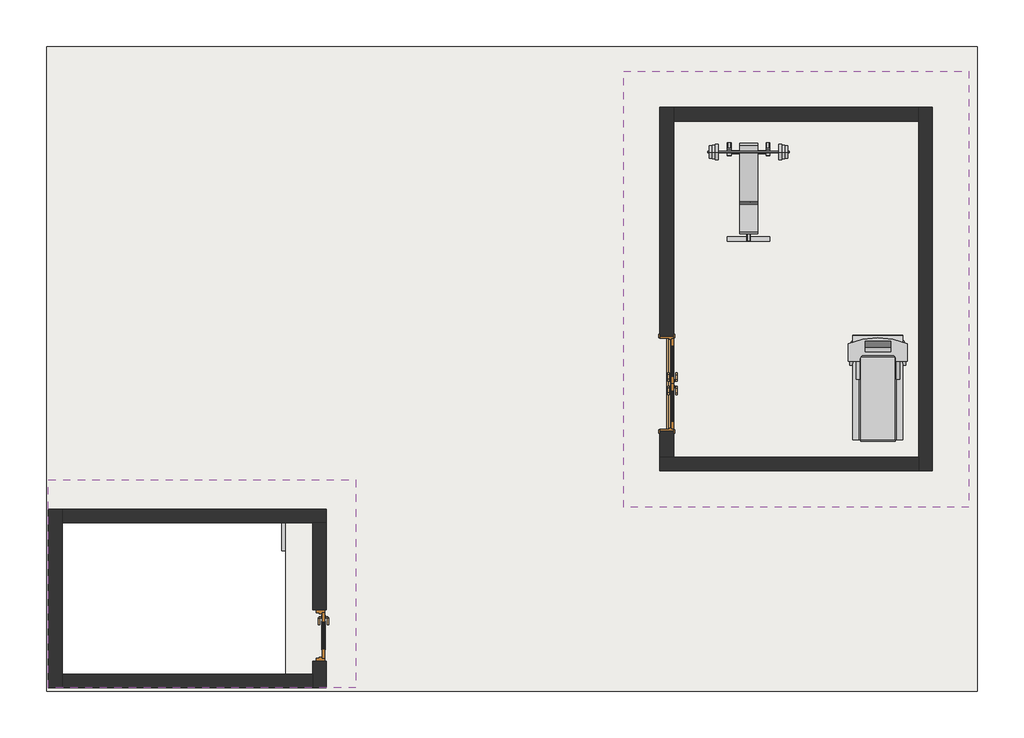
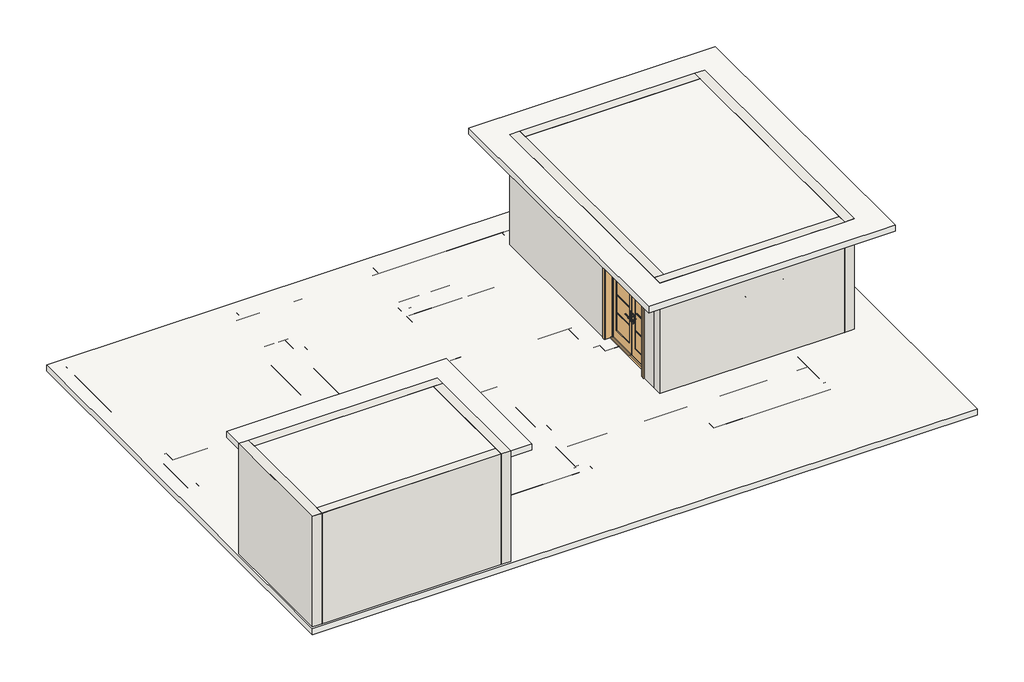
# One storey, incomplete: 18 beams, 8 walls, 3 slabs, 2 doors, 2 proxies.
"""IFC4 building model written with IfcOpenShell, lengths in millimetres."""

from ifc_helpers import new_model, si_unit, frame, origin, place, context, project, spatial, polyline, outline, extrude, faceted_brep, transform, mapped, element, save
from components import lifting_bench_lifting_bench_243d69f3, treadmill_treadmill_b3c1e061, door_7ffae4ec, door_5761e9ac

model = new_model("IFC4")

# Units and contexts
model_context = context("Model", 3, world=origin())
ifc_project = project(units=[si_unit("LENGTHUNIT", "METRE", prefix="MILLI")], contexts=[model_context])

# Site, building, storey
site = spatial("IfcSite", under=ifc_project)
building = spatial("IfcBuilding", under=site)
storey = spatial("IfcBuildingStorey", under=building, Elevation=10210.8)

# Beams
placement = place(None, origin())
element("IfcBeam", 1, ObjectType="Concrete-Rectangular Beam", at=placement, inside=storey, context=model_context, shape_type="Brep", body=[
    faceted_brep([(-8931.9263529, 6644.5661978, 10210.8), (-8931.9263529, 6415.9661978, 10210.8), (-5521.9763529, 6415.9661978, 10210.8), (-5293.3763529, 6415.9661978, 10210.8), (-2264.4263529, 6415.9661978, 10210.8), (-2035.8263529, 6415.9661978, 10210.8), (897.8736471, 6415.9661978, 10210.8), (1126.4736471, 6415.9661978, 10210.8), (3901.4236471, 6415.9661978, 10210.8), (3901.4236471, 6644.5661978, 10210.8), (1164.5736471, 6644.5661978, 10210.8), (1164.5736471, 6454.0661978, 10210.8), (859.7736471, 6454.0661978, 10210.8), (859.7736471, 6644.5661978, 10210.8), (-1997.7263529, 6644.5661978, 10210.8), (-1997.7263529, 6454.0661978, 10210.8), (-2302.5263529, 6454.0661978, 10210.8), (-2302.5263529, 6644.5661978, 10210.8), (-5198.1263529, 6644.5661978, 10210.8), (-5198.1263529, 6454.0661978, 10210.8), (-5502.9263529, 6454.0661978, 10210.8), (-5502.9263529, 6644.5661978, 10210.8), (-8931.9263529, 6415.9661978, 9906.0), (-5521.9763529, 6415.9661978, 9906.0), (-5293.3763529, 6415.9661978, 9906.0), (-2264.4263529, 6415.9661978, 9906.0), (-2035.8263529, 6415.9661978, 9906.0), (897.8736471, 6415.9661978, 9906.0), (1126.4736471, 6415.9661978, 9906.0), (3901.4236471, 6415.9661978, 9906.0), (-8931.9263529, 6644.5661978, 9906.0), (-5502.9263529, 6644.5661978, 9906.0), (-5502.9263529, 6454.0661978, 9906.0), (-5198.1263529, 6454.0661978, 9906.0), (-5198.1263529, 6644.5661978, 9906.0), (-2302.5263529, 6644.5661978, 9906.0), (-2302.5263529, 6454.0661978, 9906.0), (-1997.7263529, 6454.0661978, 9906.0), (-1997.7263529, 6644.5661978, 9906.0), (859.7736471, 6644.5661978, 9906.0), (859.7736471, 6454.0661978, 9906.0), (1164.5736471, 6454.0661978, 9906.0), (1164.5736471, 6644.5661978, 9906.0), (3901.4236471, 6644.5661978, 9906.0)], [[[0, 1, 2, 3, 4, 5, 6, 7, 8, 9, 10, 11, 12, 13, 14, 15, 16, 17, 18, 19, 20, 21]], [[1, 22, 23, 24, 25, 26, 27, 28, 29, 8, 7, 6, 5, 4, 3, 2]], [[22, 30, 31, 32, 33, 34, 35, 36, 37, 38, 39, 40, 41, 42, 43, 29, 28, 27, 26, 25, 24, 23]], [[9, 43, 42, 10]], [[1, 0, 30, 22]], [[9, 8, 29, 43]], [[33, 19, 18, 34]], [[19, 33, 32, 20]], [[20, 32, 31, 21]], [[30, 0, 21, 31]], [[37, 15, 14, 38]], [[15, 37, 36, 16]], [[16, 36, 35, 17]], [[34, 18, 17, 35]], [[41, 11, 10, 42]], [[11, 41, 40, 12]], [[12, 40, 39, 13]], [[38, 14, 13, 39]]]),
])
element("IfcBeam", 2, ObjectType="Concrete-Rectangular Beam", at=placement, inside=storey, context=model_context, shape_type="Brep", body=[
    faceted_brep([(3901.4236471, -1470.7338022, 10210.8), (4130.0236471, -1470.7338022, 10210.8), (4130.0236471, 1748.7161978, 10210.8), (3901.4236471, 1748.7161978, 10210.8), (3901.4236471, 1729.6661978, 10210.8), (3901.4236471, 34.2161978, 10210.8), (3901.4236471, -194.3838022, 10210.8), (3901.4236471, -588.0838022, 10210.8), (3901.4236471, -816.6838022, 10210.8), (3901.4236471, -1470.7338022, 9906.0), (3901.4236471, 1748.7161978, 9906.0), (3901.4236471, 1729.6661978, 9906.0), (3901.4236471, 34.2161978, 9906.0), (3901.4236471, -194.3838022, 9906.0), (3901.4236471, -588.0838022, 9906.0), (3901.4236471, -816.6838022, 9906.0), (4130.0236471, -1470.7338022, 9906.0), (4130.0236471, 1748.7161978, 9906.0)], [[[0, 1, 2, 3, 4, 5, 6, 7, 8]], [[9, 0, 8, 7, 6, 5, 4, 3, 10, 11, 12, 13, 14, 15]], [[16, 9, 15, 14, 13, 12, 11, 10, 17]], [[1, 16, 17, 2]], [[1, 0, 9, 16]], [[3, 2, 17, 10]]]),
    faceted_brep([(3901.4236471, 6377.8661978, 10210.8), (4130.0236471, 6377.8661978, 10210.8), (4130.0236471, 6377.8661978, 9906.0), (3901.4236471, 6377.8661978, 9906.0), (4130.0236471, 2053.5161978, 10210.8), (3901.4236471, 2053.5161978, 10210.8), (3901.4236471, 2053.5161978, 9906.0), (4130.0236471, 2053.5161978, 9906.0), (3901.4236471, 5558.7161978, 10210.8), (3901.4236471, 5330.1161978, 10210.8), (3901.4236471, 5044.3661978, 10210.8), (3901.4236471, 4815.7661978, 10210.8), (3901.4236471, 3012.3661978, 10210.8), (3901.4236471, 2783.7661978, 10210.8), (3901.4236471, 5558.7161978, 9906.0), (3901.4236471, 5330.1161978, 9906.0), (3901.4236471, 5044.3661978, 9906.0), (3901.4236471, 4815.7661978, 9906.0), (3901.4236471, 3012.3661978, 9906.0), (3901.4236471, 2783.7661978, 9906.0)], [[[0, 1, 2, 3]], [[4, 5, 6, 7]], [[1, 0, 8, 9, 10, 11, 12, 13, 5, 4]], [[0, 3, 14, 15, 16, 17, 18, 19, 6, 5, 13, 12, 11, 10, 9, 8]], [[3, 2, 7, 6, 19, 18, 17, 16, 15, 14]], [[2, 1, 4, 7]]]),
])
element("IfcBeam", 3, ObjectType="Concrete-Rectangular Beam", at=placement, inside=storey, context=model_context, shape_type="Brep", body=[
    faceted_brep([(3901.4236471, -1737.4338022, 10210.8), (3901.4236471, -1508.8338022, 10210.8), (-1731.0263529, -1508.8338022, 10210.8), (-1959.6263529, -1508.8338022, 10210.8), (-5293.3763529, -1508.8338022, 10210.8), (-5293.3763529, -1737.4338022, 10210.8), (-1997.7263529, -1737.4338022, 10210.8), (-1997.7263529, -1546.9338022, 10210.8), (-1692.9263529, -1546.9338022, 10210.8), (-1692.9263529, -1737.4338022, 10210.8), (859.7736471, -1737.4338022, 10210.8), (859.7736471, -1546.9338022, 10210.8), (1164.5736471, -1546.9338022, 10210.8), (1164.5736471, -1737.4338022, 10210.8), (3901.4236471, -1508.8338022, 9906.0), (-1731.0263529, -1508.8338022, 9906.0), (-1959.6263529, -1508.8338022, 9906.0), (-5293.3763529, -1508.8338022, 9906.0), (3901.4236471, -1737.4338022, 9906.0), (1164.5736471, -1737.4338022, 9906.0), (1164.5736471, -1546.9338022, 9906.0), (859.7736471, -1546.9338022, 9906.0), (859.7736471, -1737.4338022, 9906.0), (-1692.9263529, -1737.4338022, 9906.0), (-1692.9263529, -1546.9338022, 9906.0), (-1997.7263529, -1546.9338022, 9906.0), (-1997.7263529, -1737.4338022, 9906.0), (-5293.3763529, -1737.4338022, 9906.0)], [[[0, 1, 2, 3, 4, 5, 6, 7, 8, 9, 10, 11, 12, 13]], [[1, 14, 15, 16, 17, 4, 3, 2]], [[14, 18, 19, 20, 21, 22, 23, 24, 25, 26, 27, 17, 16, 15]], [[5, 27, 26, 6]], [[1, 0, 18, 14]], [[5, 4, 17, 27]], [[21, 11, 10, 22]], [[11, 21, 20, 12]], [[12, 20, 19, 13]], [[18, 0, 13, 19]], [[25, 7, 6, 26]], [[7, 25, 24, 8]], [[8, 24, 23, 9]], [[22, 10, 9, 23]]]),
])
element("IfcBeam", 4, ObjectType="Concrete-Rectangular Beam", at=placement, inside=storey, context=model_context, shape_type="Brep", body=[
    faceted_brep([(-5293.3763529, 6415.9661978, 10210.8), (-5521.9763529, 6415.9661978, 10210.8), (-5521.9763529, 3012.3661978, 10210.8), (-5521.9763529, 2783.7661978, 10210.8), (-5521.9763529, 1958.2661978, 10210.8), (-5521.9763529, 1729.6661978, 10210.8), (-5521.9763529, -327.7338022, 10210.8), (-5521.9763529, -556.3338022, 10210.8), (-5521.9763529, -1470.7338022, 10210.8), (-5293.3763529, -1470.7338022, 10210.8), (-5293.3763529, 1729.6661978, 10210.8), (-5401.3263529, 1729.6661978, 10210.8), (-5401.3263529, 1958.2661978, 10210.8), (-5293.3763529, 1958.2661978, 10210.8), (-5293.3763529, 2783.7661978, 10210.8), (-5293.3763529, 3012.3661978, 10210.8), (-5293.3763529, 5330.1161978, 10210.8), (-5293.3763529, 5558.7161978, 10210.8), (-5293.3763529, 6415.9661978, 9906.0), (-5293.3763529, 1958.2661978, 9906.0), (-5293.3763529, 2783.7661978, 9906.0), (-5293.3763529, 3012.3661978, 9906.0), (-5293.3763529, 5330.1161978, 9906.0), (-5293.3763529, 5558.7161978, 9906.0), (-5521.9763529, 6415.9661978, 9906.0), (-5401.3263529, 1958.2661978, 9906.0), (-5401.3263529, 1729.6661978, 9906.0), (-5293.3763529, 1729.6661978, 9906.0), (-5293.3763529, -1470.7338022, 9906.0), (-5521.9763529, -1470.7338022, 9906.0), (-5521.9763529, -556.3338022, 9906.0), (-5521.9763529, -327.7338022, 9906.0), (-5521.9763529, 1729.6661978, 9906.0), (-5521.9763529, 1958.2661978, 9906.0), (-5521.9763529, 2783.7661978, 9906.0), (-5521.9763529, 3012.3661978, 9906.0)], [[[0, 1, 2, 3, 4, 5, 6, 7, 8, 9, 10, 11, 12, 13, 14, 15, 16, 17]], [[18, 0, 17, 16, 15, 14, 13, 19, 20, 21, 22, 23]], [[24, 18, 23, 22, 21, 20, 19, 25, 26, 27, 28, 29, 30, 31, 32, 33, 34, 35]], [[1, 24, 35, 34, 33, 32, 31, 30, 29, 8, 7, 6, 5, 4, 3, 2]], [[1, 0, 18, 24]], [[9, 8, 29, 28]], [[12, 25, 19, 13]], [[26, 11, 10, 27]], [[11, 26, 25, 12]], [[9, 28, 27, 10]]]),
])
element("IfcBeam", 5, ObjectType="Concrete-Rectangular Beam", at=placement, inside=storey, context=model_context, shape_type="SweptSolid", body=[
    extrude(outline(polyline([(-5521.9763529, -327.7338022), (-5521.9763529, -556.3338022), (-8931.9263529, -556.3338022), (-8931.9263529, -327.7338022), (-5521.9763529, -327.7338022)])), frame((0.0, 0.0, 9906.0), z_axis=(0.0, 0.0, 1.0), x_axis=(1.0, 0.0, 0.0)), (0.0, 0.0, 1.0), 304.8),
])
element("IfcBeam", 6, ObjectType="Concrete-Rectangular Beam", at=placement, inside=storey, context=model_context, shape_type="Brep", body=[
    faceted_brep([(-9160.5263529, 6720.7661978, 10210.8), (-8931.9263529, 6720.7661978, 10210.8), (-8931.9263529, 6720.7661978, 9906.0), (-9160.5263529, 6720.7661978, 9906.0), (-9160.5263529, 6682.6661978, 10210.8), (-8931.9263529, 6682.6661978, 10210.8), (-8931.9263529, 6682.6661978, 9906.0), (-9160.5263529, 6682.6661978, 9906.0)], [[[0, 1, 2, 3]], [[1, 0, 4, 5]], [[2, 1, 5, 6]], [[3, 2, 6, 7]], [[0, 3, 7, 4]], [[5, 4, 7, 6]]]),
    faceted_brep([(-8931.9263529, 6377.8661978, 10210.8), (-9160.5263529, 6377.8661978, 10210.8), (-9160.5263529, 3050.4661978, 10210.8), (-8931.9263529, 3050.4661978, 10210.8), (-8931.9263529, 6377.8661978, 9906.0), (-8931.9263529, 3050.4661978, 9906.0), (-9160.5263529, 6377.8661978, 9906.0), (-9160.5263529, 3050.4661978, 9906.0)], [[[0, 1, 2, 3]], [[4, 0, 3, 5]], [[6, 4, 5, 7]], [[1, 6, 7, 2]], [[1, 0, 4, 6]], [[3, 2, 7, 5]]]),
    faceted_brep([(-8931.9263529, -289.6338022, 10210.8), (-9160.5263529, -289.6338022, 10210.8), (-9160.5263529, -289.6338022, 9906.0), (-8931.9263529, -289.6338022, 9906.0), (-9160.5263529, 2745.6661978, 10210.8), (-8931.9263529, 2745.6661978, 10210.8), (-8931.9263529, 2745.6661978, 9906.0), (-9160.5263529, 2745.6661978, 9906.0), (-8931.9263529, 1729.6661978, 10210.8), (-8931.9263529, 1958.2661978, 10210.8), (-8931.9263529, 1729.6661978, 9906.0), (-8931.9263529, 1958.2661978, 9906.0)], [[[0, 1, 2, 3]], [[4, 5, 6, 7]], [[1, 0, 8, 9, 5, 4]], [[0, 3, 10, 11, 6, 5, 9, 8]], [[3, 2, 7, 6, 11, 10]], [[2, 1, 4, 7]]]),
])
element("IfcBeam", 7, ObjectType="Concrete-Rectangular Beam", at=placement, inside=storey, context=model_context, shape_type="Brep", body=[
    faceted_brep([(-8931.9263529, 3012.3661978, 10210.8), (-8931.9263529, 2783.7661978, 10210.8), (-5521.9763529, 2783.7661978, 10210.8), (-5521.9763529, 3012.3661978, 10210.8), (-8931.9263529, 2783.7661978, 9906.0), (-5521.9763529, 2783.7661978, 9906.0), (-8931.9263529, 3012.3661978, 9906.0), (-5521.9763529, 3012.3661978, 9906.0)], [[[0, 1, 2, 3]], [[1, 4, 5, 2]], [[4, 6, 7, 5]], [[6, 0, 3, 7]], [[1, 0, 6, 4]], [[3, 2, 5, 7]]]),
    faceted_brep([(3901.4236471, 3012.3661978, 10210.8), (3901.4236471, 2783.7661978, 10210.8), (3901.4236471, 2783.7661978, 9906.0), (3901.4236471, 3012.3661978, 9906.0), (-5293.3763529, 2783.7661978, 10210.8), (-5293.3763529, 3012.3661978, 10210.8), (-5293.3763529, 3012.3661978, 9906.0), (-5293.3763529, 2783.7661978, 9906.0), (1126.4736471, 3012.3661978, 10210.8), (897.8736471, 3012.3661978, 10210.8), (-2035.8263529, 3012.3661978, 10210.8), (-2264.4263529, 3012.3661978, 10210.8), (-4601.2263529, 3012.3661978, 10210.8), (-4829.8263529, 3012.3661978, 10210.8), (351.7736471, 2783.7661978, 10210.8), (580.3736471, 2783.7661978, 10210.8), (1977.3736471, 2783.7661978, 10210.8), (2205.9736471, 2783.7661978, 10210.8), (351.7736471, 2783.7661978, 9906.0), (580.3736471, 2783.7661978, 9906.0), (1977.3736471, 2783.7661978, 9906.0), (2205.9736471, 2783.7661978, 9906.0), (-4829.8263529, 3012.3661978, 9906.0), (-4601.2263529, 3012.3661978, 9906.0), (-2264.4263529, 3012.3661978, 9906.0), (-2035.8263529, 3012.3661978, 9906.0), (897.8736471, 3012.3661978, 9906.0), (1126.4736471, 3012.3661978, 9906.0)], [[[0, 1, 2, 3]], [[4, 5, 6, 7]], [[1, 0, 8, 9, 10, 11, 12, 13, 5, 4, 14, 15, 16, 17]], [[2, 1, 17, 16, 15, 14, 4, 7, 18, 19, 20, 21]], [[3, 2, 21, 20, 19, 18, 7, 6, 22, 23, 24, 25, 26, 27]], [[0, 3, 27, 26, 25, 24, 23, 22, 6, 5, 13, 12, 11, 10, 9, 8]]]),
])
element("IfcBeam", 8, ObjectType="Concrete-Rectangular Beam", at=placement, inside=storey, context=model_context, shape_type="Brep", body=[
    faceted_brep([(-8931.9263529, 1958.2661978, 10210.8), (-8931.9263529, 1729.6661978, 10210.8), (-5521.9763529, 1729.6661978, 10210.8), (-5521.9763529, 1958.2661978, 10210.8), (-8931.9263529, 1729.6661978, 9906.0), (-5521.9763529, 1729.6661978, 9906.0), (-8931.9263529, 1958.2661978, 9906.0), (-5521.9763529, 1958.2661978, 9906.0)], [[[0, 1, 2, 3]], [[1, 4, 5, 2]], [[4, 6, 7, 5]], [[6, 0, 3, 7]], [[1, 0, 6, 4]], [[3, 2, 5, 7]]]),
    faceted_brep([(3901.4236471, 1958.2661978, 10210.8), (3901.4236471, 1748.7161978, 10210.8), (3901.4236471, 1729.6661978, 10210.8), (3901.4236471, 1729.6661978, 9906.0), (3901.4236471, 1748.7161978, 9906.0), (3901.4236471, 1958.2661978, 9906.0), (618.4736471, 1729.6661978, 10210.8), (618.4736471, 1958.2661978, 10210.8), (618.4736471, 1958.2661978, 9906.0), (618.4736471, 1729.6661978, 9906.0), (2205.9736471, 1958.2661978, 10210.8), (1977.3736471, 1958.2661978, 10210.8), (1977.3736471, 1958.2661978, 9906.0), (2205.9736471, 1958.2661978, 9906.0)], [[[0, 1, 2, 3, 4, 5]], [[6, 7, 8, 9]], [[2, 1, 0, 10, 11, 7, 6]], [[3, 2, 6, 9]], [[5, 4, 3, 9, 8, 12, 13]], [[0, 5, 13, 12, 8, 7, 11, 10]]]),
    faceted_brep([(-5096.5263529, 1958.2661978, 10210.8), (-5096.5263529, 1729.6661978, 10210.8), (-1959.6263529, 1729.6661978, 10210.8), (-1731.0263529, 1729.6661978, 10210.8), (313.6736471, 1729.6661978, 10210.8), (313.6736471, 1958.2661978, 10210.8), (-5096.5263529, 1729.6661978, 9906.0), (-1959.6263529, 1729.6661978, 9906.0), (-1731.0263529, 1729.6661978, 9906.0), (313.6736471, 1729.6661978, 9906.0), (-5096.5263529, 1958.2661978, 9906.0), (313.6736471, 1958.2661978, 9906.0)], [[[0, 1, 2, 3, 4, 5]], [[1, 6, 7, 8, 9, 4, 3, 2]], [[6, 10, 11, 9, 8, 7]], [[10, 0, 5, 11]], [[1, 0, 10, 6]], [[5, 4, 9, 11]]]),
])
element("IfcBeam", 9, ObjectType="Concrete-Rectangular Beam", at=placement, inside=storey, context=model_context, shape_type="Brep", body=[
    faceted_brep([(-1959.6263529, -1508.8338022, 10210.8), (-1731.0263529, -1508.8338022, 10210.8), (-1731.0263529, -816.6838022, 10210.8), (-1731.0263529, -588.0838022, 10210.8), (-1731.0263529, -194.3838022, 10210.8), (-1731.0263529, 34.2161978, 10210.8), (-1731.0263529, 1729.6661978, 10210.8), (-1959.6263529, 1729.6661978, 10210.8), (-1959.6263529, -1508.8338022, 9906.0), (-1959.6263529, 1729.6661978, 9906.0), (-1731.0263529, -1508.8338022, 9906.0), (-1731.0263529, 1729.6661978, 9906.0), (-1731.0263529, 34.2161978, 9906.0), (-1731.0263529, -194.3838022, 9906.0), (-1731.0263529, -588.0838022, 9906.0), (-1731.0263529, -816.6838022, 9906.0)], [[[0, 1, 2, 3, 4, 5, 6, 7]], [[8, 0, 7, 9]], [[10, 8, 9, 11, 12, 13, 14, 15]], [[1, 10, 15, 14, 13, 12, 11, 6, 5, 4, 3, 2]], [[1, 0, 8, 10]], [[7, 6, 11, 9]]]),
])
element("IfcBeam", 10, ObjectType="Concrete-Rectangular Beam", at=placement, inside=storey, context=model_context, shape_type="SweptSolid", body=[
    extrude(outline(polyline([(3901.4236471, -588.0838022), (3901.4236471, -816.6838022), (-1731.0263529, -816.6838022), (-1731.0263529, -588.0838022), (3901.4236471, -588.0838022)])), frame((0.0, 0.0, 9906.0), z_axis=(0.0, 0.0, 1.0), x_axis=(1.0, 0.0, 0.0)), (0.0, 0.0, 1.0), 304.8),
])
element("IfcBeam", 11, ObjectType="Concrete-Rectangular Beam", at=placement, inside=storey, context=model_context, shape_type="SweptSolid", body=[
    extrude(outline(polyline([(3901.4236471, 34.2161978), (3901.4236471, -194.3838022), (-1731.0263529, -194.3838022), (-1731.0263529, 34.2161978), (3901.4236471, 34.2161978)])), frame((0.0, 0.0, 9906.0), z_axis=(0.0, 0.0, 1.0), x_axis=(1.0, 0.0, 0.0)), (0.0, 0.0, 1.0), 304.8),
])
element("IfcBeam", 12, ObjectType="Concrete-Rectangular Beam", at=placement, inside=storey, context=model_context, shape_type="Brep", body=[
    faceted_brep([(3901.4236471, 5330.1161978, 10210.8), (3901.4236471, 5558.7161978, 10210.8), (1126.4736471, 5558.7161978, 10210.8), (897.8736471, 5558.7161978, 10210.8), (-2035.8263529, 5558.7161978, 10210.8), (-2264.4263529, 5558.7161978, 10210.8), (-5293.3763529, 5558.7161978, 10210.8), (-5293.3763529, 5330.1161978, 10210.8), (-4829.8263529, 5330.1161978, 10210.8), (-4601.2263529, 5330.1161978, 10210.8), (-2264.4263529, 5330.1161978, 10210.8), (-2035.8263529, 5330.1161978, 10210.8), (897.8736471, 5330.1161978, 10210.8), (1126.4736471, 5330.1161978, 10210.8), (3901.4236471, 5330.1161978, 9906.0), (-5293.3763529, 5330.1161978, 9906.0), (-4829.8263529, 5330.1161978, 9906.0), (-4601.2263529, 5330.1161978, 9906.0), (-2264.4263529, 5330.1161978, 9906.0), (-2035.8263529, 5330.1161978, 9906.0), (897.8736471, 5330.1161978, 9906.0), (1126.4736471, 5330.1161978, 9906.0), (3901.4236471, 5558.7161978, 9906.0), (-5293.3763529, 5558.7161978, 9906.0), (-2264.4263529, 5558.7161978, 9906.0), (-2035.8263529, 5558.7161978, 9906.0), (897.8736471, 5558.7161978, 9906.0), (1126.4736471, 5558.7161978, 9906.0)], [[[0, 1, 2, 3, 4, 5, 6, 7, 8, 9, 10, 11, 12, 13]], [[14, 0, 13, 12, 11, 10, 9, 8, 7, 15, 16, 17, 18, 19, 20, 21]], [[22, 14, 21, 20, 19, 18, 17, 16, 15, 23, 24, 25, 26, 27]], [[1, 22, 27, 26, 25, 24, 23, 6, 5, 4, 3, 2]], [[1, 0, 14, 22]], [[7, 6, 23, 15]]]),
])
element("IfcBeam", 13, ObjectType="Concrete-Rectangular Beam", at=placement, inside=storey, context=model_context, shape_type="Brep", body=[
    faceted_brep([(3901.4236471, 4815.7661978, 10210.8), (3901.4236471, 5044.3661978, 10210.8), (1126.4736471, 5044.3661978, 10210.8), (897.8736471, 5044.3661978, 10210.8), (-2035.8263529, 5044.3661978, 10210.8), (-2264.4263529, 5044.3661978, 10210.8), (-4601.2263529, 5044.3661978, 10210.8), (-4601.2263529, 4815.7661978, 10210.8), (-2264.4263529, 4815.7661978, 10210.8), (-2035.8263529, 4815.7661978, 10210.8), (897.8736471, 4815.7661978, 10210.8), (1126.4736471, 4815.7661978, 10210.8), (3901.4236471, 4815.7661978, 9906.0), (-4601.2263529, 4815.7661978, 9906.0), (-2264.4263529, 4815.7661978, 9906.0), (-2035.8263529, 4815.7661978, 9906.0), (897.8736471, 4815.7661978, 9906.0), (1126.4736471, 4815.7661978, 9906.0), (3901.4236471, 5044.3661978, 9906.0), (-4601.2263529, 5044.3661978, 9906.0), (-2264.4263529, 5044.3661978, 9906.0), (-2035.8263529, 5044.3661978, 9906.0), (897.8736471, 5044.3661978, 9906.0), (1126.4736471, 5044.3661978, 9906.0)], [[[0, 1, 2, 3, 4, 5, 6, 7, 8, 9, 10, 11]], [[12, 0, 11, 10, 9, 8, 7, 13, 14, 15, 16, 17]], [[18, 12, 17, 16, 15, 14, 13, 19, 20, 21, 22, 23]], [[1, 18, 23, 22, 21, 20, 19, 6, 5, 4, 3, 2]], [[1, 0, 12, 18]], [[7, 6, 19, 13]]]),
])
element("IfcBeam", 14, ObjectType="Concrete-Rectangular Beam", at=placement, inside=storey, context=model_context, shape_type="Brep", body=[
    faceted_brep([(-4829.8263529, 3012.3661978, 10210.8), (-4601.2263529, 3012.3661978, 10210.8), (-4601.2263529, 4815.7661978, 10210.8), (-4601.2263529, 5044.3661978, 10210.8), (-4601.2263529, 5330.1161978, 10210.8), (-4829.8263529, 5330.1161978, 10210.8), (-4829.8263529, 3012.3661978, 9906.0), (-4829.8263529, 5330.1161978, 9906.0), (-4601.2263529, 3012.3661978, 9906.0), (-4601.2263529, 5330.1161978, 9906.0), (-4601.2263529, 5044.3661978, 9906.0), (-4601.2263529, 4815.7661978, 9906.0)], [[[0, 1, 2, 3, 4, 5]], [[6, 0, 5, 7]], [[8, 6, 7, 9, 10, 11]], [[1, 8, 11, 10, 9, 4, 3, 2]], [[1, 0, 6, 8]], [[5, 4, 9, 7]]]),
])
element("IfcBeam", 15, ObjectType="Concrete-Rectangular Beam", at=placement, inside=storey, context=model_context, shape_type="SweptSolid", body=[
    extrude(outline(polyline([(-2035.8263529, 3012.3661978), (-2264.4263529, 3012.3661978), (-2264.4263529, 4815.7661978), (-2035.8263529, 4815.7661978), (-2035.8263529, 3012.3661978)])), frame((0.0, 0.0, 9906.0), z_axis=(0.0, 0.0, 1.0), x_axis=(1.0, 0.0, 0.0)), (0.0, 0.0, 1.0), 304.8),
    extrude(outline(polyline([(-2264.4263529, 6415.9661978), (-2035.8263529, 6415.9661978), (-2035.8263529, 5558.7161978), (-2264.4263529, 5558.7161978), (-2264.4263529, 6415.9661978)])), frame((0.0, 0.0, 9906.0), z_axis=(0.0, 0.0, 1.0), x_axis=(1.0, 0.0, 0.0)), (0.0, 0.0, 1.0), 304.8),
    extrude(outline(polyline([(-2264.4263529, 5330.1161978), (-2035.8263529, 5330.1161978), (-2035.8263529, 5044.3661978), (-2264.4263529, 5044.3661978), (-2264.4263529, 5330.1161978)])), frame((0.0, 0.0, 9906.0), z_axis=(0.0, 0.0, 1.0), x_axis=(1.0, 0.0, 0.0)), (0.0, 0.0, 1.0), 304.8),
])
element("IfcBeam", 16, ObjectType="Concrete-Rectangular Beam", at=placement, inside=storey, context=model_context, shape_type="SweptSolid", body=[
    extrude(outline(polyline([(1126.4736471, 3012.3661978), (897.8736471, 3012.3661978), (897.8736471, 4815.7661978), (1126.4736471, 4815.7661978), (1126.4736471, 3012.3661978)])), frame((0.0, 0.0, 9906.0), z_axis=(0.0, 0.0, 1.0), x_axis=(1.0, 0.0, 0.0)), (0.0, 0.0, 1.0), 304.8),
    extrude(outline(polyline([(897.8736471, 6415.9661978), (1126.4736471, 6415.9661978), (1126.4736471, 5558.7161978), (897.8736471, 5558.7161978), (897.8736471, 6415.9661978)])), frame((0.0, 0.0, 9906.0), z_axis=(0.0, 0.0, 1.0), x_axis=(1.0, 0.0, 0.0)), (0.0, 0.0, 1.0), 304.8),
    extrude(outline(polyline([(897.8736471, 5330.1161978), (1126.4736471, 5330.1161978), (1126.4736471, 5044.3661978), (897.8736471, 5044.3661978), (897.8736471, 5330.1161978)])), frame((0.0, 0.0, 9906.0), z_axis=(0.0, 0.0, 1.0), x_axis=(1.0, 0.0, 0.0)), (0.0, 0.0, 1.0), 304.8),
])
element("IfcBeam", 17, ObjectType="Concrete-Rectangular Beam", at=placement, inside=storey, context=model_context, shape_type="SweptSolid", body=[
    extrude(outline(polyline([(351.7736471, 2783.7661978), (580.3736471, 2783.7661978), (580.3736471, 1958.2661978), (351.7736471, 1958.2661978), (351.7736471, 2783.7661978)])), frame((0.0, 0.0, 9906.0), z_axis=(0.0, 0.0, 1.0), x_axis=(1.0, 0.0, 0.0)), (0.0, 0.0, 1.0), 304.8),
])
element("IfcBeam", 18, ObjectType="Concrete-Rectangular Beam", at=placement, inside=storey, context=model_context, shape_type="SweptSolid", body=[
    extrude(outline(polyline([(1977.3736471, 2783.7661978), (2205.9736471, 2783.7661978), (2205.9736471, 1958.2661978), (1977.3736471, 1958.2661978), (1977.3736471, 2783.7661978)])), frame((0.0, 0.0, 9906.0), z_axis=(0.0, 0.0, 1.0), x_axis=(1.0, 0.0, 0.0)), (0.0, 0.0, 1.0), 304.8),
])

# Proxies
lifting_bench_lifting_bench_shape = lifting_bench_lifting_bench_243d69f3(model_context)
element("IfcBuildingElementProxy", 19, Name="Lifting Bench : Lifting Bench", ObjectType="Lifting Bench : Lifting Bench", at=placement, inside=storey, context=model_context, shape_type="MappedRepresentation", body=[
    mapped(lifting_bench_lifting_bench_shape, transform((1954.8382003, 3718.5744906, 10210.8), x_axis=(1.0, 0.0, 0.0), y_axis=(0.0, 1.0, 0.0), z_axis=(0.0, 0.0, 1.0))),
])
treadmill_treadmill_shape = treadmill_treadmill_b3c1e061(model_context)
element("IfcBuildingElementProxy", 20, Name="Treadmill : Treadmill", ObjectType="Treadmill : Treadmill", at=placement, inside=storey, context=model_context, shape_type="MappedRepresentation", body=[
    mapped(treadmill_treadmill_shape, transform((4035.8856165, 2143.7744906, 10210.8), x_axis=(1.0, 0.0, 0.0), y_axis=(0.0, 1.0, 0.0), z_axis=(0.0, 0.0, 1.0))),
])

# Doors
door_shape = door_7ffae4ec(model_context)
element("IfcDoor", 21, ObjectType="Door-Exterior-Double-Full Glass-Wood_Clad : 60\" x 84\"", at=placement, inside=storey, context=model_context, shape_type="MappedRepresentation", body=[
    mapped(door_shape, transform((940.2606165, 1330.9744906, 10210.8), x_axis=(0.0, -1.0, 0.0), y_axis=(1.0, 0.0, 0.0), z_axis=(0.0, 0.0, 1.0))),
])
door_2_shape = door_5761e9ac(model_context)
element("IfcDoor", 22, ObjectType="Door-Passage-Single-Full_Lite : 30\" x 84\"", at=placement, inside=storey, context=model_context, shape_type="MappedRepresentation", body=[
    mapped(door_2_shape, transform((-4893.3263529, -2893.1338022, 10210.8), x_axis=(0.0, -1.0, 0.0), y_axis=(1.0, 0.0, 0.0), z_axis=(0.0, 0.0, 1.0))),
])

# Slabs
element("IfcSlab", 23, ObjectType="Generic - 6\"", at=placement, inside=storey, context=model_context, shape_type="SweptSolid", body=[
    extrude(outline(polyline([(6149.3236471, 6987.4661978), (6149.3236471, -3826.5838022), (-9465.3263529, -3826.5838022), (-9465.3263529, 6987.4661978), (6149.3236471, 6987.4661978)]), holes=[polyline([(-5458.4763529, -1000.8338022), (-9204.9763529, -1000.8338022), (-9204.9763529, -3540.8338022), (-5458.4763529, -3540.8338022), (-5458.4763529, -1000.8338022)])]), frame((0.0, 0.0, 10058.4), z_axis=(0.0, 0.0, 1.0), x_axis=(1.0, 0.0, 0.0)), (0.0, 0.0, 1.0), 152.4),
])
element("IfcSlab", 24, ObjectType="Generic - 6\"", at=placement, inside=storey, context=model_context, shape_type="SweptSolid", body=[
    extrude(outline(polyline([(-4277.3763529, -3769.4338022), (-9433.5763529, -3769.4338022), (-9433.5763529, -276.9338022), (-4277.3763529, -276.9338022), (-4277.3763529, -3769.4338022)])), frame((0.0, 0.0, 12801.6), z_axis=(0.0, 0.0, 1.0), x_axis=(1.0, 0.0, 0.0)), (0.0, 0.0, 1.0), 152.4),
])
element("IfcSlab", 25, ObjectType="Generic - 6\"", at=placement, inside=storey, context=model_context, shape_type="SweptSolid", body=[
    extrude(outline(polyline([(6004.3856165, 6576.0744906), (6004.3856165, -739.1255094), (213.1856165, -739.1255094), (213.1856165, 6576.0744906), (6004.3856165, 6576.0744906)])), frame((0.0, 0.0, 12801.6), z_axis=(0.0, 0.0, 1.0), x_axis=(1.0, 0.0, 0.0)), (0.0, 0.0, 1.0), 152.4),
])

# Walls
element("IfcWall", 26, ObjectType="Generic - 9\"", at=placement, inside=storey, context=model_context, shape_type="Brep", body=[
    faceted_brep([(-9433.5763529, -772.2338022, 10210.8), (-9433.5763529, -3769.4338022, 10210.8), (-9433.5763529, -3769.4338022, 12954.0), (-9433.5763529, -772.2338022, 12954.0), (-9204.9763529, -772.2338022, 10210.8), (-9204.9763529, -772.2338022, 12954.0), (-9204.9763529, -1000.8338022, 12954.0), (-9204.9763529, -3540.8338022, 12954.0), (-9204.9763529, -3769.4338022, 12954.0), (-9204.9763529, -3769.4338022, 10210.8), (-9204.9763529, -3540.8338022, 10210.8), (-9204.9763529, -1000.8338022, 10210.8)], [[[0, 1, 2, 3]], [[4, 5, 6, 7, 8, 9, 10, 11]], [[1, 0, 4, 11, 10, 9]], [[3, 2, 8, 7, 6, 5]], [[2, 1, 9, 8]], [[0, 3, 5, 4]]]),
])
element("IfcWall", 27, ObjectType="Generic - 9\"", at=placement, inside=storey, context=model_context, shape_type="SweptSolid", body=[
    extrude(outline(polyline([(-5001.2763529, -3769.4338022), (-9204.9763529, -3769.4338022), (-9204.9763529, -3540.8338022), (-5001.2763529, -3540.8338022), (-5001.2763529, -3769.4338022)])), frame((0.0, 0.0, 10210.8), z_axis=(0.0, 0.0, 1.0), x_axis=(1.0, 0.0, 0.0)), (0.0, 0.0, 1.0), 2743.2),
])
element("IfcWall", 28, ObjectType="Generic - 9\"", at=placement, inside=storey, context=model_context, shape_type="Brep", body=[
    faceted_brep([(-9204.9763529, -1000.8338022, 10210.8), (-5001.2763529, -1000.8338022, 10210.8), (-4772.6763529, -1000.8338022, 10210.8), (-4772.6763529, -1000.8338022, 12954.0), (-5001.2763529, -1000.8338022, 12954.0), (-9204.9763529, -1000.8338022, 12954.0), (-9204.9763529, -772.2338022, 10210.8), (-9204.9763529, -772.2338022, 12954.0), (-4772.6763529, -772.2338022, 12954.0), (-4772.6763529, -772.2338022, 10210.8)], [[[0, 1, 2, 3, 4, 5]], [[6, 7, 8, 9]], [[2, 1, 0, 6, 9]], [[5, 4, 3, 8, 7]], [[0, 5, 7, 6]], [[3, 2, 9, 8]]]),
])
element("IfcWall", 29, ObjectType="Generic - 9\"", at=placement, inside=storey, context=model_context, shape_type="Brep", body=[
    faceted_brep([(-5001.2763529, -3769.4338022, 12954.0), (-5001.2763529, -3540.8338022, 12954.0), (-5001.2763529, -1000.8338022, 12954.0), (-5001.2763529, -1000.8338022, 10210.8), (-5001.2763529, -2461.3338022, 10210.8), (-5001.2763529, -2461.3338022, 12446.0), (-5001.2763529, -3324.9338022, 12446.0), (-5001.2763529, -3324.9338022, 10210.8), (-5001.2763529, -3540.8338022, 10210.8), (-5001.2763529, -3769.4338022, 10210.8), (-4772.6763529, -1000.8338022, 12954.0), (-4772.6763529, -3769.4338022, 12954.0), (-4772.6763529, -3769.4338022, 10210.8), (-4772.6763529, -3324.9338022, 10210.8), (-4772.6763529, -3324.9338022, 12446.0), (-4772.6763529, -2461.3338022, 12446.0), (-4772.6763529, -2461.3338022, 10210.8), (-4772.6763529, -1000.8338022, 10210.8)], [[[0, 1, 2, 3, 4, 5, 6, 7, 8, 9]], [[10, 11, 12, 13, 14, 15, 16, 17]], [[3, 17, 16, 4]], [[12, 9, 8, 7, 13]], [[2, 1, 0, 11, 10]], [[3, 2, 10, 17]], [[0, 9, 12, 11]], [[6, 14, 13, 7]], [[14, 6, 5, 15]], [[15, 5, 4, 16]]]),
])
element("IfcWall", 30, ObjectType="Generic - 9\"", at=placement, inside=storey, context=model_context, shape_type="Brep", body=[
    faceted_brep([(5166.1856165, 5966.4744906, 10210.8), (5166.1856165, 5737.8744906, 10210.8), (5166.1856165, 99.0744906, 10210.8), (5166.1856165, -129.5255094, 10210.8), (5166.1856165, -129.5255094, 12954.0), (5166.1856165, 99.0744906, 12954.0), (5166.1856165, 5737.8744906, 12954.0), (5166.1856165, 5966.4744906, 12954.0), (5394.7856165, 5966.4744906, 10210.8), (5394.7856165, 5966.4744906, 12954.0), (5394.7856165, -129.5255094, 12954.0), (5394.7856165, -129.5255094, 10210.8)], [[[0, 1, 2, 3, 4, 5, 6, 7]], [[8, 9, 10, 11]], [[3, 2, 1, 0, 8, 11]], [[7, 6, 5, 4, 10, 9]], [[4, 3, 11, 10]], [[0, 7, 9, 8]]]),
])
element("IfcWall", 31, ObjectType="Generic - 9\"", at=placement, inside=storey, context=model_context, shape_type="Brep", body=[
    faceted_brep([(5166.1856165, 99.0744906, 10210.8), (1051.3856165, 99.0744906, 10210.8), (822.7856165, 99.0744906, 10210.8), (822.7856165, 99.0744906, 12954.0), (1051.3856165, 99.0744906, 12954.0), (5166.1856165, 99.0744906, 12954.0), (5166.1856165, -129.5255094, 10210.8), (5166.1856165, -129.5255094, 12954.0), (822.7856165, -129.5255094, 12954.0), (822.7856165, -129.5255094, 10210.8)], [[[0, 1, 2, 3, 4, 5]], [[6, 7, 8, 9]], [[2, 1, 0, 6, 9]], [[5, 4, 3, 8, 7]], [[0, 5, 7, 6]], [[3, 2, 9, 8]]]),
])
element("IfcWall", 32, ObjectType="Generic - 9\"", at=placement, inside=storey, context=model_context, shape_type="Brep", body=[
    faceted_brep([(1051.3856165, 5966.4744906, 12954.0), (1051.3856165, 5737.8744906, 12954.0), (1051.3856165, 99.0744906, 12954.0), (1051.3856165, 99.0744906, 10210.8), (1051.3856165, 543.5744906, 10210.8), (1051.3856165, 543.5744906, 12369.8), (1051.3856165, 2118.3744906, 12369.8), (1051.3856165, 2118.3744906, 10210.8), (1051.3856165, 5737.8744906, 10210.8), (1051.3856165, 5966.4744906, 10210.8), (822.7856165, 99.0744906, 12954.0), (822.7856165, 5966.4744906, 12954.0), (822.7856165, 5966.4744906, 10210.8), (822.7856165, 2118.3744906, 10210.8), (822.7856165, 2118.3744906, 12369.8), (822.7856165, 543.5744906, 12369.8), (822.7856165, 543.5744906, 10210.8), (822.7856165, 99.0744906, 10210.8)], [[[0, 1, 2, 3, 4, 5, 6, 7, 8, 9]], [[10, 11, 12, 13, 14, 15, 16, 17]], [[3, 17, 16, 4]], [[12, 9, 8, 7, 13]], [[2, 1, 0, 11, 10]], [[3, 2, 10, 17]], [[0, 9, 12, 11]], [[15, 5, 4, 16]], [[5, 15, 14, 6]], [[6, 14, 13, 7]]]),
])
element("IfcWall", 33, ObjectType="Generic - 9\"", at=placement, inside=storey, context=model_context, shape_type="SweptSolid", body=[
    extrude(outline(polyline([(5166.1856165, 5737.8744906), (1051.3856165, 5737.8744906), (1051.3856165, 5966.4744906), (5166.1856165, 5966.4744906), (5166.1856165, 5737.8744906)])), frame((0.0, 0.0, 10210.8), z_axis=(0.0, 0.0, 1.0), x_axis=(1.0, 0.0, 0.0)), (0.0, 0.0, 1.0), 2743.2),
])

save(model, "model.ifc")

# Revit data of these elements
# Type "Concrete-Rectangular Beam"
#   Assembly Code = "B10"
#   Length [instance default] = 5' - 0"
#   b = 0' - 9"
#   h = 1' - 0"
#   Structural Material [instance default] = Concrete, Cast-in-Place gray
# Type "Lifting Bench : Lifting Bench"
#   Assembly Code = "E1090"
#   Default Elevation = 0
# Type "Treadmill : Treadmill"
#   Assembly Code = "E1090"
#   Default Elevation = 0
# Type "Door-Exterior-Double-Full Glass-Wood_Clad : 60\" x 84\""
#   Type Mark = "18"
#   Assembly Code = "B2030100"
#   Analytic Construction = "French door, wood frame with double glass"
#   Top Rail = 0' - 4 11/16"
#   Threshold Offset [instance default] = 0' - 0 1/2"
#   Thickness = 0' - 1 3/8"
#   Thermal Resistance (R) = 1.9158 (h·ft²·°F)/BTU
#   Swing Angle [instance default] = 90.00°
#   Stiles = 0' - 4 3/4"
#   Rough Width = 5' - 2"
#   Rough Height = 7' - 1"
#   Panel Width = 2' - 6"
#   Door Offset [instance default] = 0' - 0"
#   Height = 7' - 0"
#   Width = 5' - 0"
#   Heat Transfer Coefficient (U) = 0.5220 BTU/(h·ft²·°F)
#   Bottom Rail = 0' - 9 1/8"
#   Exterior Trim [instance default] = yes
#   Threshold [instance default] = yes
#   Show Grill [instance default] = yes
#   Function = 1
#   Trim Material = Cherry
#   Threshold Material = Cherry
#   Panel Material = Cherry
#   Glazing = Glass
#   Frame Material = Cherry
#   Door Handle Material = Aluminum
#   Visual Light Transmittance = 0
#   Solar Heat Gain Coefficient = 0
#   Wall Closure = (empty or 0)
#   Construction Type = (empty or 0)
# Type "Door-Passage-Single-Full_Lite : 30\" x 84\""
#   Type Mark = "11"
#   Assembly Code = "B2030100"
#   Analytic Construction = "Wooden"
#   Thickness = 0' - 1 3/4"
#   Thermal Resistance (R) = 2.5876 (h·ft²·°F)/BTU
#   Swing Angle [instance default] = 90.00°
#   Strike Height = 3' - 4"
#   Rough Width [instance default] = 2' - 10"
#   Rough Height [instance default] = 7' - 4"
#   MF Opening Height [instance default] = 0' - 4"
#   MF Opening Width [instance default] = 0' - 4"
#   Inset Calculate [instance default] = 0' - 4"
#   Masonry Inset [instance default] = 0' - 1"
#   Height = 7' - 0"
#   Width = 2' - 6"
#   Heat Transfer Coefficient (U) = 0.3865 BTU/(h·ft²·°F)
#   Masonry Frame Depth = 0' - 5 3/4"
#   Masonry Frame [instance default] = yes
#   Function = 1
#   Dry Wall Frame [instance default] = no
#   Panel Material = Wood - Birch
#   Glazing = Glass
#   Glass Stop Material = Metal - Paint Finish - Grey
#   Frame Material = Metal - Paint Finish - Grey
#   Door Handle Material = Aluminum
#   Visual Light Transmittance = 0
#   Solar Heat Gain Coefficient = 0
#   Wall Closure = (empty or 0)
# Type "Generic - 6\""
#   Assembly Code = "B1010"
#   Function = 0
#   Layers, outside or top first: 0' - 6" no material (function 1)
# Type "Generic - 9\""
#   Assembly Code = "B2010"
#   Layers, outside or top first: 0' - 9" no material (function 1)
# Elements 1, 2, 3, 4, 5, 6, 7, 8, 9, 10, 11, 12, 13, 14, 15, 16, 17, 18 (IfcBeam, "Concrete-Rectangular Beam")
#   Structural Material = Concrete, Cast-in-Place gray
#   Phase Created = New Construction
#   Materials on its faces: "Concrete, Cast-in-Place gray"
# Element 19 (IfcBuildingElementProxy, "Lifting Bench : Lifting Bench")
#   Phase Created = New Construction
#   Materials on its faces: "Plastic - Black"
# Element 20 (IfcBuildingElementProxy, "Treadmill : Treadmill")
#   Phase Created = New Construction
#   Materials on its faces: "Metal - Steel"
# Element 21 (IfcDoor, "Door-Exterior-Double-Full Glass-Wood_Clad : 60\" x 84\"")
#   Threshold Offset = 0' - 0 1/2"
#   Swing Angle = 90.00°
#   Door Offset = 0' - 0"
#   Threshold = yes
#   Show Grill = yes
#   Exterior Trim = yes
#   Phase Created = New Construction
#   Materials on its faces: "Cherry", "Aluminum", "Glass"
# Element 22 (IfcDoor, "Door-Passage-Single-Full_Lite : 30\" x 84\"")
#   Swing Angle = 90.00°
#   Rough Width = 2' - 10"
#   Rough Height = 7' - 4"
#   Masonry Inset = 0' - 1"
#   MF Opening Width = 0' - 4"
#   MF Opening Height = 0' - 4"
#   Inset Calculate = 0' - 4"
#   Masonry Frame = yes
#   Dry Wall Frame = no
#   Phase Created = New Construction
#   Materials on its faces: "Metal - Paint Finish - Grey", "Aluminum", "Wood - Birch", "Glass"
# Element 23 (IfcSlab, "Generic - 6\"")
#   Height Offset From Level = 0' - 0"
#   Phase Created = New Construction
#   Materials on its faces: "Default Floor"
# Elements 24, 25 (IfcSlab, "Generic - 6\"")
#   Height Offset From Level = 9' - 0"
#   Phase Created = New Construction
#   Materials on its faces: "Default Floor"
# Elements 26, 27, 28, 29, 30, 31, 32, 33 (IfcWall, "Generic - 9\"")
#   Top Offset = 0' - 0"
#   Base Offset = 0' - 0"
#   Unconnected Height = 9' - 0"
#   wall height = 9' - 0"
#   Phase Created = New Construction
#   Materials on its faces: "Default Wall"
# Materials
#   "Concrete, Cast-in-Place gray": class "Concrete", colour RGB 192 192 192, transparency 0, Description = "Cast-in-place concrete", Cost = 0
#   "Cherry": class "Wood", colour RGB 226 177 128, transparency 0, Description = "Prunus Serotina", Cost = 0
#   "Glass": class "Glass", colour RGB 0 128 192, transparency 0.75, Description = "Soda Lime Glass", Cost = 0
#   "Aluminum": class "Metal", colour RGB 247 247 247, transparency 0, Description = "Aluminum 6061", Cost = 0
#   "Wood - Birch": class "Wood", colour RGB 166 116 52, transparency 0, Cost = 0
#   "Metal - Paint Finish - Grey": class "Paint", colour RGB 104 104 104, transparency 0, Cost = 0
#   "Plastic - Black": colour RGB 0 0 0, transparency 0
#   "Metal - Steel": colour RGB 210 210 210, transparency 0
#   "Default Floor": colour RGB 128 128 128, transparency 0, Cost = 0
#   "Default Wall": colour RGB 128 128 128, transparency 0, Cost = 0
